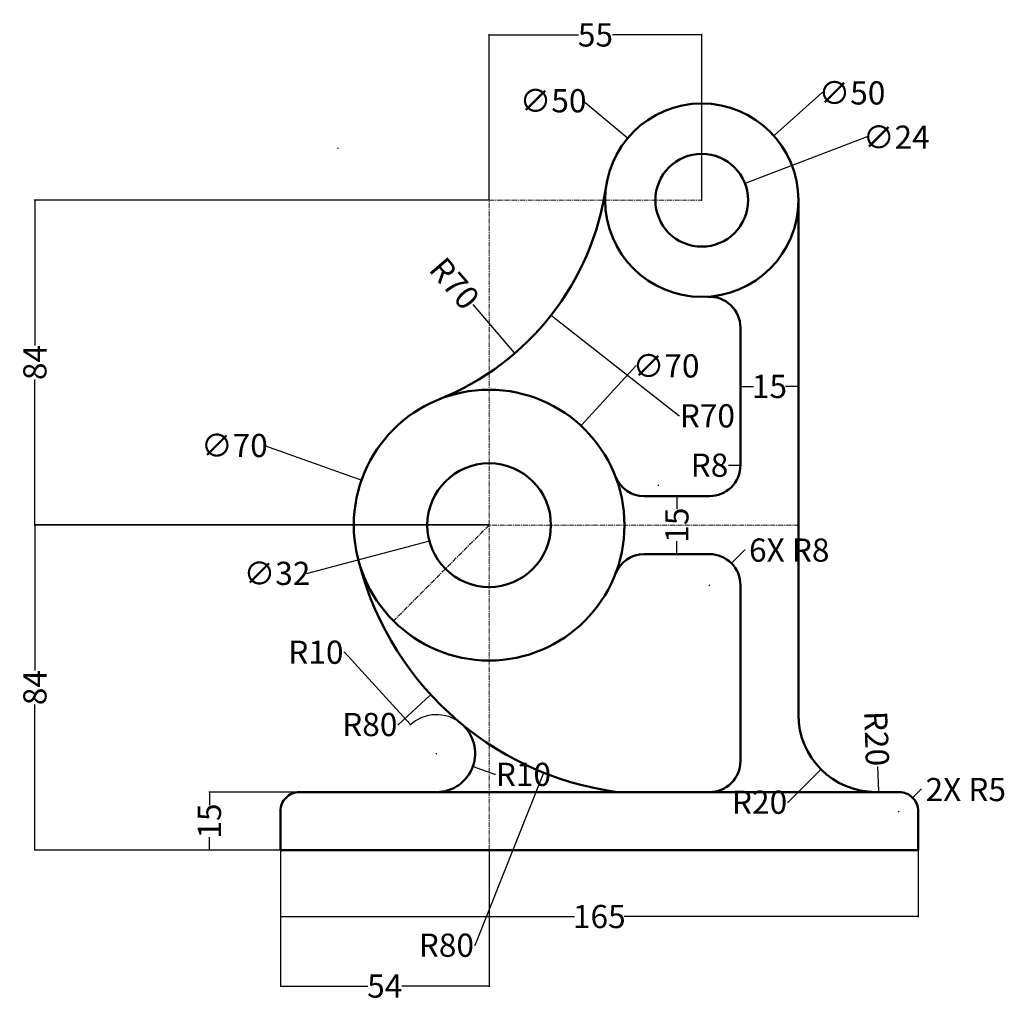
# Model space of a CAD drawing. Units: millimetres. Extents: x -55 to 200, y -2 to 251.
import ezdxf

# ---------------------------------------------------------------- set-up
doc = ezdxf.new("R2010")
doc.units = ezdxf.units.MM
doc.header["$MEASUREMENT"] = 0
doc.linetypes.add('CENTER', pattern=[2, 1.25, -0.25, 0.25, -0.25])
for name, color, linetype, lineweight in [('M-CNTR', 4, 'CENTER', 18), ('M-DIMS', 2, 'Continuous', 25), ('M-OUTL', 7, 'Continuous', 50)]:
    doc.layers.add(name, color=color, linetype=linetype, lineweight=lineweight)
doc.styles.get("Standard").update_dxf_attribs({"font": 'arial.ttf'})
doc.dimstyles.get("Standard").update_dxf_attribs({"dimtxt": 6, "dimasz": 0.18, "dimexe": 0.18, "dimexo": 0.0625, "dimgap": 0.09, "dimtad": 0, "dimtoh": 1, "dimdec": 0, "dimzin": 0, "dimdsep": 46, "dimtxsty": 'Standard', "dimcen": 0.09, "dimadec": 0, "dimazin": 0, "dimtfac": 1, "dimtdec": 0, "dimtofl": 0, "dimtmove": 0, "dimatfit": 3, "dimfxl": 1, "dimtolj": 1, "dimtzin": 0, "dimarcsym": 0})

# ---------------------------------------------------------------- blocks, each defined once
blk = doc.blocks.new('*D1')
at = {"layer": 'Defpoints', "color": 0, "transparency": 16777216}
for p in [(12.77, 36.84), (66.77, 36.84), (66.77, 1.69)]:
    blk.add_point(p, dxfattribs=at)
at = {"layer": 'M-DIMS', "color": 0, "lineweight": -2, "transparency": 16777216}
for p, q in [((12.77, 36.77), (12.77, 1.51)), ((66.77, 36.77), (66.77, 1.51)), ((12.95, 1.69), (35.4, 1.69)), ((66.59, 1.69), (44.15, 1.69))]:
    blk.add_line(p, q, dxfattribs=at)
at = {"layer": 'M-DIMS', "color": 0, "transparency": 16777216}
for points in [[(12.95, 1.72), (12.95, 1.66), (12.77, 1.69)], [(66.59, 1.72), (66.59, 1.66), (66.77, 1.69)]]:
    blk.add_solid(points, dxfattribs=at)
at = {"layer": 'M-DIMS', "color": 0, "transparency": 16777216, "insert": (39.77, 1.69), "char_height": 6, "attachment_point": 5}
blk.add_mtext('\\A1;54', dxfattribs=at)
blk = doc.blocks.new('*D2')
at = {"layer": 'Defpoints', "color": 0, "transparency": 16777216}
for p in [(123.77, 136.34), (131.77, 136.34)]:
    blk.add_point(p, dxfattribs=at)
at = {"layer": 'M-DIMS', "color": 0, "lineweight": -2, "transparency": 16777216}
blk.add_line((128.71, 136.34), (131.59, 136.34), dxfattribs=at)
blk.add_arc((123.77, 136.34), 8, 0.4476, 1.2892, dxfattribs=at)
at = {"layer": 'M-DIMS', "color": 0, "transparency": 16777216}
blk.add_solid([(131.59, 136.37), (131.59, 136.31), (131.77, 136.34)], dxfattribs=at)
at = {"layer": 'M-DIMS', "color": 0, "transparency": 16777216, "insert": (123.77, 136.34), "char_height": 6, "attachment_point": 5}
blk.add_mtext('\\A1;R8', dxfattribs=at)
blk = doc.blocks.new('*D3')
at = {"layer": 'Defpoints', "color": 0, "transparency": 16777216}
for p in [(27.73, 218.31), (73.38, 165.24)]:
    blk.add_point(p, dxfattribs=at)
at = {"layer": 'M-DIMS', "color": 0, "lineweight": -2, "transparency": 16777216}
blk.add_line((62.55, 177.84), (73.27, 165.38), dxfattribs=at)
at = {"layer": 'M-DIMS', "color": 0, "transparency": 16777216}
blk.add_solid([(73.29, 165.4), (73.24, 165.36), (73.38, 165.24)], dxfattribs=at)
at = {"layer": 'M-DIMS', "color": 0, "transparency": 16777216, "insert": (57.82, 183.33), "char_height": 6, "attachment_point": 5, "rotation": 310.7032}
blk.add_mtext('\\A1;R70', dxfattribs=at)
blk = doc.blocks.new('*D4')
at = {"layer": 'Defpoints', "color": 0, "transparency": 16777216}
for p in [(110.59, 131.13), (51.69, 76.99)]:
    blk.add_point(p, dxfattribs=at)
at = {"layer": 'M-DIMS', "color": 0, "lineweight": -2, "transparency": 16777216}
for p, q in [((110.5, 131.13), (110.68, 131.13)), ((110.59, 131.04), (110.59, 131.22)), ((43.33, 69.3), (51.56, 76.87)), ((43.15, 69.3), (43.33, 69.3))]:
    blk.add_line(p, q, dxfattribs=at)
at = {"layer": 'M-DIMS', "color": 0, "transparency": 16777216}
blk.add_solid([(51.54, 76.89), (51.58, 76.85), (51.69, 76.99)], dxfattribs=at)
at = {"layer": 'M-DIMS', "color": 0, "transparency": 16777216, "insert": (35.9, 69.3), "char_height": 6, "attachment_point": 5}
blk.add_mtext('\\A1;R80', dxfattribs=at)
blk = doc.blocks.new('*D5')
at = {"layer": 'Defpoints', "color": 0, "transparency": 16777216}
for p in [(46.43, 69.24), (53.16, 61.84)]:
    blk.add_point(p, dxfattribs=at)
at = {"layer": 'M-DIMS', "color": 0, "lineweight": -2, "transparency": 16777216}
for p, q in [((29.2, 87.99), (29.38, 87.99)), ((29.38, 87.99), (46.31, 69.37)), ((53.07, 61.84), (53.25, 61.84)), ((53.16, 61.75), (53.16, 61.93))]:
    blk.add_line(p, q, dxfattribs=at)
blk.add_arc((53.16, 61.84), 10, 50.7056, 133.3049, dxfattribs=at)
at = {"layer": 'M-DIMS', "color": 0, "transparency": 16777216}
blk.add_solid([(46.33, 69.39), (46.29, 69.35), (46.43, 69.24)], dxfattribs=at)
at = {"layer": 'M-DIMS', "color": 0, "transparency": 16777216, "insert": (21.96, 87.99), "char_height": 6, "attachment_point": 5}
blk.add_mtext('\\A1;R10', dxfattribs=at)
blk = doc.blocks.new('*D6')
at = {"layer": 'Defpoints', "color": 0, "transparency": 16777216}
for p in [(82.24, 124.92), (51.3, 116.75)]:
    blk.add_point(p, dxfattribs=at)
at = {"layer": 'M-DIMS', "color": 0, "lineweight": -2, "transparency": 16777216}
for p, q in [((66.68, 120.84), (66.86, 120.84)), ((66.77, 120.75), (66.77, 120.93)), ((19.52, 108.37), (51.13, 116.71))]:
    blk.add_line(p, q, dxfattribs=at)
at = {"layer": 'M-DIMS', "color": 0, "transparency": 16777216}
blk.add_solid([(51.12, 116.74), (51.14, 116.68), (51.3, 116.75)], dxfattribs=at)
at = {"layer": 'M-DIMS', "color": 0, "transparency": 16777216, "insert": (11.9, 108.37), "char_height": 6, "attachment_point": 5}
blk.add_mtext('\\A1;∅32', dxfattribs=at)
blk = doc.blocks.new('*D7')
at = {"layer": 'Defpoints', "color": 0, "transparency": 16777216}
for p in [(33.79, 132.53), (99.76, 109.14)]:
    blk.add_point(p, dxfattribs=at)
at = {"layer": 'M-DIMS', "color": 0, "lineweight": -2, "transparency": 16777216}
for p, q in [((8.52, 141.43), (8.7, 141.43)), ((8.7, 141.43), (33.62, 132.59)), ((66.68, 120.84), (66.86, 120.84)), ((66.77, 120.75), (66.77, 120.93))]:
    blk.add_line(p, q, dxfattribs=at)
at = {"layer": 'M-DIMS', "color": 0, "transparency": 16777216}
blk.add_solid([(33.63, 132.62), (33.61, 132.56), (33.79, 132.53)], dxfattribs=at)
at = {"layer": 'M-DIMS', "color": 0, "transparency": 16777216, "insert": (0.88, 141.43), "char_height": 6, "attachment_point": 5}
blk.add_mtext('\\A1;∅70', dxfattribs=at)
blk = doc.blocks.new('*D8')
at = {"layer": 'Defpoints', "color": 0, "transparency": 16777216}
for p in [(132.98, 209.13), (110.57, 200.54)]:
    blk.add_point(p, dxfattribs=at)
at = {"layer": 'M-DIMS', "color": 0, "lineweight": -2, "transparency": 16777216}
for p, q in [((164.28, 221.13), (133.15, 209.2)), ((164.46, 221.13), (164.28, 221.13)), ((121.68, 204.84), (121.86, 204.84)), ((121.77, 204.75), (121.77, 204.93))]:
    blk.add_line(p, q, dxfattribs=at)
at = {"layer": 'M-DIMS', "color": 0, "transparency": 16777216}
blk.add_solid([(133.14, 209.22), (133.16, 209.17), (132.98, 209.13)], dxfattribs=at)
at = {"layer": 'M-DIMS', "color": 0, "transparency": 16777216, "insert": (172.1, 221.13), "char_height": 6, "attachment_point": 5}
blk.add_mtext('\\A1;∅24', dxfattribs=at)
blk = doc.blocks.new('*D9')
at = {"layer": 'Defpoints', "color": 0, "transparency": 16777216}
for p in [(140.41, 221.5), (103.14, 188.17)]:
    blk.add_point(p, dxfattribs=at)
at = {"layer": 'M-DIMS', "color": 0, "lineweight": -2, "transparency": 16777216}
for p, q in [((152.81, 232.58), (140.55, 221.62)), ((152.99, 232.58), (152.81, 232.58)), ((121.68, 204.84), (121.86, 204.84)), ((121.77, 204.75), (121.77, 204.93))]:
    blk.add_line(p, q, dxfattribs=at)
at = {"layer": 'M-DIMS', "color": 0, "transparency": 16777216}
blk.add_solid([(140.53, 221.64), (140.57, 221.59), (140.41, 221.5)], dxfattribs=at)
at = {"layer": 'M-DIMS', "color": 0, "transparency": 16777216, "insert": (160.63, 232.58), "char_height": 6, "attachment_point": 5}
blk.add_mtext('\\A1;∅50', dxfattribs=at)
blk = doc.blocks.new('*D10')
at = {"layer": 'Defpoints', "color": 0, "transparency": 16777216}
for p in [(166.77, 71.84), (167.51, 51.85)]:
    blk.add_point(p, dxfattribs=at)
at = {"layer": 'M-DIMS', "color": 0, "lineweight": -2, "transparency": 16777216}
blk.add_line((167.27, 58.43), (167.51, 52.03), dxfattribs=at)
blk.add_arc((166.77, 71.84), 20, 270.179, 272.6379, dxfattribs=at)
at = {"layer": 'M-DIMS', "color": 0, "transparency": 16777216}
blk.add_solid([(167.54, 52.03), (167.48, 52.03), (167.51, 51.85)], dxfattribs=at)
at = {"layer": 'M-DIMS', "color": 0, "transparency": 16777216, "insert": (167, 65.67), "char_height": 6, "attachment_point": 5, "rotation": 272.1222}
blk.add_mtext('\\A1;R20', dxfattribs=at)
blk = doc.blocks.new('*D11')
at = {"layer": 'Defpoints', "color": 0, "transparency": 16777216}
for p in [(115.33, 128.34), (115.33, 113.34), (115.33, 113.34)]:
    blk.add_point(p, dxfattribs=at)
at = {"layer": 'M-DIMS', "color": 0, "lineweight": -2, "transparency": 16777216}
for p, q in [((115.33, 128.16), (115.33, 124.96)), ((115.39, 128.34), (115.51, 128.34)), ((115.33, 113.52), (115.33, 116.71)), ((115.39, 113.34), (115.51, 113.34))]:
    blk.add_line(p, q, dxfattribs=at)
at = {"layer": 'M-DIMS', "color": 0, "transparency": 16777216}
for points in [[(115.3, 128.16), (115.36, 128.16), (115.33, 128.34)], [(115.3, 113.52), (115.36, 113.52), (115.33, 113.34)]]:
    blk.add_solid(points, dxfattribs=at)
at = {"layer": 'M-DIMS', "color": 0, "transparency": 16777216, "insert": (115.33, 120.84), "char_height": 6, "attachment_point": 5, "rotation": 90}
blk.add_mtext('\\A1;15', dxfattribs=at)
blk = doc.blocks.new('*D12')
at = {"layer": 'Defpoints', "color": 0, "transparency": 16777216}
for p in [(131.77, 171.9), (146.77, 172.16), (146.77, 156.71)]:
    blk.add_point(p, dxfattribs=at)
at = {"layer": 'M-DIMS', "color": 0, "lineweight": -2, "transparency": 16777216}
for p, q in [((131.77, 171.83), (131.77, 156.53)), ((146.77, 172.1), (146.77, 156.53)), ((131.95, 156.71), (135.15, 156.71)), ((146.59, 156.71), (143.4, 156.71))]:
    blk.add_line(p, q, dxfattribs=at)
at = {"layer": 'M-DIMS', "color": 0, "transparency": 16777216}
for points in [[(131.95, 156.74), (131.95, 156.68), (131.77, 156.71)], [(146.59, 156.74), (146.59, 156.68), (146.77, 156.71)]]:
    blk.add_solid(points, dxfattribs=at)
at = {"layer": 'M-DIMS', "color": 0, "transparency": 16777216, "insert": (139.27, 156.71), "char_height": 6, "attachment_point": 5}
blk.add_mtext('\\A1;15', dxfattribs=at)
blk = doc.blocks.new('*D13')
at = {"layer": 'Defpoints', "color": 0, "transparency": 16777216}
for p in [(12.77, 36.84), (177.77, 36.84), (177.77, 19.67)]:
    blk.add_point(p, dxfattribs=at)
at = {"layer": 'M-DIMS', "color": 0, "lineweight": -2, "transparency": 16777216}
for p, q in [((12.77, 36.77), (12.77, 19.49)), ((177.77, 36.77), (177.77, 19.49)), ((12.95, 19.67), (88.82, 19.67)), ((177.59, 19.67), (101.73, 19.67))]:
    blk.add_line(p, q, dxfattribs=at)
at = {"layer": 'M-DIMS', "color": 0, "transparency": 16777216}
for points in [[(12.95, 19.7), (12.95, 19.64), (12.77, 19.67)], [(177.59, 19.7), (177.59, 19.64), (177.77, 19.67)]]:
    blk.add_solid(points, dxfattribs=at)
at = {"layer": 'M-DIMS', "color": 0, "transparency": 16777216, "insert": (95.27, 19.67), "char_height": 6, "attachment_point": 5}
blk.add_mtext('\\A1;165', dxfattribs=at)
blk = doc.blocks.new('*D14')
at = {"layer": 'Defpoints', "color": 0, "transparency": 16777216}
for p in [(-50.72, 120.84), (66.86, 120.84), (66.77, 36.84)]:
    blk.add_point(p, dxfattribs=at)
at = {"layer": 'M-DIMS', "color": 0, "lineweight": -2, "transparency": 16777216}
for p, q in [((66.8, 120.84), (-50.9, 120.84)), ((-50.72, 120.66), (-50.72, 83.22)), ((-50.72, 37.02), (-50.72, 74.46)), ((66.71, 36.84), (-50.9, 36.84))]:
    blk.add_line(p, q, dxfattribs=at)
at = {"layer": 'M-DIMS', "color": 0, "transparency": 16777216}
for points in [[(-50.75, 120.66), (-50.69, 120.66), (-50.72, 120.84)], [(-50.75, 37.02), (-50.69, 37.02), (-50.72, 36.84)]]:
    blk.add_solid(points, dxfattribs=at)
at = {"layer": 'M-DIMS', "color": 0, "transparency": 16777216, "insert": (-50.72, 78.84), "char_height": 6, "attachment_point": 5, "rotation": 90}
blk.add_mtext('\\A1;84', dxfattribs=at)
blk = doc.blocks.new('*D15')
at = {"layer": 'Defpoints', "color": 0, "transparency": 16777216}
for p in [(-50.72, 204.84), (66.77, 204.84), (66.77, 120.93)]:
    blk.add_point(p, dxfattribs=at)
at = {"layer": 'M-DIMS', "color": 0, "lineweight": -2, "transparency": 16777216}
for p, q in [((66.71, 204.84), (-50.9, 204.84)), ((-50.72, 204.66), (-50.72, 167.26)), ((-50.72, 121.11), (-50.72, 158.5)), ((66.71, 120.93), (-50.9, 120.93))]:
    blk.add_line(p, q, dxfattribs=at)
at = {"layer": 'M-DIMS', "color": 0, "transparency": 16777216}
for points in [[(-50.75, 204.66), (-50.69, 204.66), (-50.72, 204.84)], [(-50.75, 121.11), (-50.69, 121.11), (-50.72, 120.93)]]:
    blk.add_solid(points, dxfattribs=at)
at = {"layer": 'M-DIMS', "color": 0, "transparency": 16777216, "insert": (-50.72, 162.88), "char_height": 6, "attachment_point": 5, "rotation": 90}
blk.add_mtext('\\A1;84', dxfattribs=at)
blk = doc.blocks.new('*D16')
at = {"layer": 'Defpoints', "color": 0, "transparency": 16777216}
for p in [(121.77, 247.56), (66.77, 204.84), (121.77, 204.93)]:
    blk.add_point(p, dxfattribs=at)
at = {"layer": 'M-DIMS', "color": 0, "lineweight": -2, "transparency": 16777216}
for p, q in [((66.77, 204.9), (66.77, 247.74)), ((66.95, 247.56), (89.86, 247.56)), ((121.59, 247.56), (98.68, 247.56)), ((121.77, 204.99), (121.77, 247.74))]:
    blk.add_line(p, q, dxfattribs=at)
at = {"layer": 'M-DIMS', "color": 0, "transparency": 16777216}
for points in [[(66.95, 247.59), (66.95, 247.53), (66.77, 247.56)], [(121.59, 247.59), (121.59, 247.53), (121.77, 247.56)]]:
    blk.add_solid(points, dxfattribs=at)
at = {"layer": 'M-DIMS', "color": 0, "transparency": 16777216, "insert": (94.27, 247.56), "char_height": 6, "attachment_point": 5}
blk.add_mtext('\\A1;55', dxfattribs=at)
blk = doc.blocks.new('*D17')
at = {"layer": 'Defpoints', "color": 0, "transparency": 16777216}
for p in [(-5.58, 51.84), (17.77, 51.84), (12.77, 36.84)]:
    blk.add_point(p, dxfattribs=at)
at = {"layer": 'M-DIMS', "color": 0, "lineweight": -2, "transparency": 16777216}
for p, q in [((17.71, 51.84), (-5.76, 51.84)), ((-5.58, 51.66), (-5.58, 48.46)), ((-5.58, 37.02), (-5.58, 40.21)), ((12.71, 36.84), (-5.76, 36.84))]:
    blk.add_line(p, q, dxfattribs=at)
at = {"layer": 'M-DIMS', "color": 0, "transparency": 16777216}
for points in [[(-5.61, 51.66), (-5.55, 51.66), (-5.58, 51.84)], [(-5.61, 37.02), (-5.55, 37.02), (-5.58, 36.84)]]:
    blk.add_solid(points, dxfattribs=at)
at = {"layer": 'M-DIMS', "color": 0, "transparency": 16777216, "insert": (-5.58, 44.34), "char_height": 6, "attachment_point": 5, "rotation": 90}
blk.add_mtext('\\A1;15', dxfattribs=at)
blk = doc.blocks.new('*D18')
at = {"layer": 'Defpoints', "color": 0, "transparency": 16777216}
for p in [(90.5, 146.57), (43.05, 95.1)]:
    blk.add_point(p, dxfattribs=at)
at = {"layer": 'M-DIMS', "color": 0, "lineweight": -2, "transparency": 16777216}
for p, q in [((104.73, 162.01), (90.62, 146.7)), ((104.91, 162.01), (104.73, 162.01)), ((66.68, 120.84), (66.86, 120.84)), ((66.77, 120.75), (66.77, 120.93))]:
    blk.add_line(p, q, dxfattribs=at)
at = {"layer": 'M-DIMS', "color": 0, "transparency": 16777216}
blk.add_solid([(90.6, 146.72), (90.64, 146.68), (90.5, 146.57)], dxfattribs=at)
at = {"layer": 'M-DIMS', "color": 0, "transparency": 16777216, "insert": (112.55, 162.01), "char_height": 6, "attachment_point": 5}
blk.add_mtext('\\A1;∅70', dxfattribs=at)
blk = doc.blocks.new('*D19')
at = {"layer": 'Defpoints', "color": 0, "transparency": 16777216}
for p in [(102.62, 220.91), (140.92, 188.77)]:
    blk.add_point(p, dxfattribs=at)
at = {"layer": 'M-DIMS', "color": 0, "lineweight": -2, "transparency": 16777216}
for p, q in [((90.95, 230.55), (91.13, 230.55)), ((91.13, 230.55), (102.49, 221.02)), ((121.68, 204.84), (121.86, 204.84)), ((121.77, 204.75), (121.77, 204.93))]:
    blk.add_line(p, q, dxfattribs=at)
at = {"layer": 'M-DIMS', "color": 0, "transparency": 16777216}
blk.add_solid([(102.5, 221.04), (102.47, 221), (102.62, 220.91)], dxfattribs=at)
at = {"layer": 'M-DIMS', "color": 0, "transparency": 16777216, "insert": (83.31, 230.55), "char_height": 6, "attachment_point": 5}
blk.add_mtext('\\A1;∅50', dxfattribs=at)
blk = doc.blocks.new('*D20')
at = {"layer": 'Defpoints', "color": 0, "transparency": 16777216}
for p in [(110.59, 131.13), (80.93, 56.83)]:
    blk.add_point(p, dxfattribs=at)
at = {"layer": 'M-DIMS', "color": 0, "lineweight": -2, "transparency": 16777216}
for p, q in [((110.5, 131.13), (110.68, 131.13)), ((110.59, 131.04), (110.59, 131.22)), ((63.14, 12.25), (80.87, 56.66)), ((62.96, 12.25), (63.14, 12.25))]:
    blk.add_line(p, q, dxfattribs=at)
at = {"layer": 'M-DIMS', "color": 0, "transparency": 16777216}
blk.add_solid([(80.84, 56.67), (80.89, 56.65), (80.93, 56.83)], dxfattribs=at)
at = {"layer": 'M-DIMS', "color": 0, "transparency": 16777216, "insert": (55.71, 12.25), "char_height": 6, "attachment_point": 5}
blk.add_mtext('\\A1;R80', dxfattribs=at)
blk = doc.blocks.new('*D21')
at = {"layer": 'Defpoints', "color": 0, "transparency": 16777216}
for p in [(27.73, 218.31), (82.77, 175.06)]:
    blk.add_point(p, dxfattribs=at)
at = {"layer": 'M-DIMS', "color": 0, "lineweight": -2, "transparency": 16777216}
for p, q in [((27.64, 218.31), (27.82, 218.31)), ((27.73, 218.22), (27.73, 218.4)), ((115.8, 149.1), (82.91, 174.94)), ((115.98, 149.1), (115.8, 149.1))]:
    blk.add_line(p, q, dxfattribs=at)
at = {"layer": 'M-DIMS', "color": 0, "transparency": 16777216}
blk.add_solid([(82.93, 174.97), (82.9, 174.92), (82.77, 175.06)], dxfattribs=at)
at = {"layer": 'M-DIMS', "color": 0, "transparency": 16777216, "insert": (123.22, 149.1), "char_height": 6, "attachment_point": 5}
blk.add_mtext('\\A1;R70', dxfattribs=at)
blk = doc.blocks.new('*D22')
at = {"layer": 'Defpoints', "color": 0, "transparency": 16777216}
for p in [(166.77, 71.84), (152.63, 57.69)]:
    blk.add_point(p, dxfattribs=at)
at = {"layer": 'M-DIMS', "color": 0, "lineweight": -2, "transparency": 16777216}
for p, q in [((166.68, 71.84), (166.86, 71.84)), ((166.77, 71.75), (166.77, 71.93)), ((144.15, 49.21), (152.5, 57.57)), ((143.97, 49.21), (144.15, 49.21))]:
    blk.add_line(p, q, dxfattribs=at)
at = {"layer": 'M-DIMS', "color": 0, "transparency": 16777216}
blk.add_solid([(152.48, 57.59), (152.53, 57.55), (152.63, 57.69)], dxfattribs=at)
at = {"layer": 'M-DIMS', "color": 0, "transparency": 16777216, "insert": (136.72, 49.21), "char_height": 6, "attachment_point": 5}
blk.add_mtext('\\A1;R20', dxfattribs=at)
blk = doc.blocks.new('*D23')
at = {"layer": 'Defpoints', "color": 0, "transparency": 16777216}
for p in [(53.16, 61.84), (62.56, 58.44)]:
    blk.add_point(p, dxfattribs=at)
at = {"layer": 'M-DIMS', "color": 0, "lineweight": -2, "transparency": 16777216}
for p, q in [((53.07, 61.84), (53.25, 61.84)), ((53.16, 61.75), (53.16, 61.93)), ((68.21, 56.41), (62.73, 58.38)), ((68.39, 56.41), (68.21, 56.41))]:
    blk.add_line(p, q, dxfattribs=at)
at = {"layer": 'M-DIMS', "color": 0, "transparency": 16777216}
blk.add_solid([(62.74, 58.41), (62.72, 58.35), (62.56, 58.44)], dxfattribs=at)
at = {"layer": 'M-DIMS', "color": 0, "transparency": 16777216, "insert": (75.64, 56.41), "char_height": 6, "attachment_point": 5}
blk.add_mtext('\\A1;R10', dxfattribs=at)
blk = doc.blocks.new('*D24')
at = {"layer": 'Defpoints', "color": 0, "transparency": 16777216}
for p in [(129.43, 110.99), (123.77, 105.34)]:
    blk.add_point(p, dxfattribs=at)
at = {"layer": 'M-DIMS', "color": 0, "lineweight": -2, "transparency": 16777216}
for p, q in [((132.83, 114.39), (129.56, 111.12)), ((133.01, 114.39), (132.83, 114.39)), ((123.68, 105.34), (123.86, 105.34)), ((123.77, 105.25), (123.77, 105.43))]:
    blk.add_line(p, q, dxfattribs=at)
at = {"layer": 'M-DIMS', "color": 0, "transparency": 16777216}
blk.add_solid([(129.54, 111.14), (129.58, 111.1), (129.43, 110.99)], dxfattribs=at)
at = {"layer": 'M-DIMS', "color": 0, "transparency": 16777216, "insert": (144.4, 114.39), "char_height": 6, "attachment_point": 5}
blk.add_mtext('\\A1;6X R8', dxfattribs=at)
blk = doc.blocks.new('*D25')
at = {"layer": 'Defpoints', "color": 0, "transparency": 16777216}
for p in [(176.31, 50.37), (172.77, 46.84)]:
    blk.add_point(p, dxfattribs=at)
at = {"layer": 'M-DIMS', "color": 0, "lineweight": -2, "transparency": 16777216}
for p, q in [((178.43, 52.49), (176.44, 50.5)), ((178.61, 52.49), (178.43, 52.49)), ((172.68, 46.84), (172.86, 46.84)), ((172.77, 46.75), (172.77, 46.93))]:
    blk.add_line(p, q, dxfattribs=at)
at = {"layer": 'M-DIMS', "color": 0, "transparency": 16777216}
blk.add_solid([(176.42, 50.52), (176.46, 50.48), (176.31, 50.37)], dxfattribs=at)
at = {"layer": 'M-DIMS', "color": 0, "transparency": 16777216, "insert": (190.06, 52.49), "char_height": 6, "attachment_point": 5}
blk.add_mtext('\\A1;2X R5', dxfattribs=at)

msp = doc.modelspace()

# ---------------------------------------------------------------- linework, layer by layer
at = {"layer": 'M-CNTR'}
for points in [[(66.77, 19.14), (66.77, 36.84), (66.77, 120.84), (66.77, 204.84), (121.77, 204.84)], [(146.77, 120.84), (66.77, 120.84), (42.03, 96.09)]]:
    msp.add_lwpolyline(points, dxfattribs=at)
at = {"layer": 'M-OUTL'}
msp.add_line((146.77, 204.84), (146.77, 71.84), dxfattribs=at)
for points in [[(131.77, 136.34), (131.77, 171.9, 0.432089), (123.29, 179.88)], [(99.42, 133.45, 0.309892), (106.88, 128.34), (123.77, 128.34, 0.414214), (131.77, 136.34)], [(131.77, 105.34, 0.414214), (123.77, 113.34), (106.88, 113.34, 0.309892), (99.42, 108.22)], [(123.77, 51.84, 0.414214), (131.77, 59.84), (131.77, 105.34)]]:
    msp.add_lwpolyline(points, format="xyb", dxfattribs=at)
msp.add_lwpolyline([(177.77, 36.84), (177.77, 46.84, 0.414214), (172.77, 51.84), (166.77, 51.84), (17.77, 51.84, 0.414214), (12.77, 46.84), (12.77, 36.84)], format="xyb", close=True, dxfattribs=at)
for centre, radius in [((121.77, 204.84), 25), ((121.77, 204.84), 12), ((66.77, 120.84), 35), ((66.77, 120.84), 16)]:
    msp.add_circle(centre, radius, dxfattribs=at)
for centre, radius, start, end in [((27.73, 218.31), 70, 291.8272, 351.8471), ((110.59, 131.13), 80, 192.5253, 262.3803), ((166.77, 71.84), 20, 180, 270), ((53.16, 61.84), 10, 270, 50.3475)]:
    msp.add_arc(centre, radius, start, end, dxfattribs=at)

# ---------------------------------------------------------------- dimensions: what is measured, and where the dimension line sits
at = {"layer": 'M-DIMS'}
for base, p1, p2, picture, middle in [((121.77, 247.56), (66.77, 204.84), (121.77, 204.93), '*D16', (94.27, 247.56)), ((146.77, 156.71), (131.77, 171.9), (146.77, 172.16), '*D12', (139.27, 156.71)), ((66.77, 1.69), (12.77, 36.84), (66.77, 36.84), '*D1', (39.77, 1.69)), ((177.77, 19.67), (12.77, 36.84), (177.77, 36.84), '*D13', (95.27, 19.67))]:
    dim = msp.add_linear_dim(base=base, p1=p1, p2=p2, dimstyle='Standard', override={"dimclrd": 0, "dimclre": 0, "dimclrt": 0}, dxfattribs=at)
    dim.commit()
    dim.dimension.update_dxf_attribs({"geometry": picture, "text_midpoint": middle})
for p1, p2, override, picture, middle in [((140.92, 188.77), (102.62, 220.91), {"dimdec": 0, "dimlfac": 1, "dimrnd": 0, "dimzin": 0, "dimdsep": 46, "dimlunit": 2}, '*D19', (83.31, 230.55)), ((103.14, 188.17), (140.41, 221.5), {"dimclrd": 0, "dimclre": 0, "dimclrt": 0}, '*D9', (160.63, 232.58)), ((110.57, 200.54), (132.98, 209.13), {"dimclrd": 0, "dimclre": 0, "dimclrt": 0}, '*D8', (172.1, 221.13)), ((43.05, 95.1), (90.5, 146.57), {"dimdec": 0, "dimlfac": 1, "dimrnd": 0, "dimzin": 0, "dimdsep": 46, "dimlunit": 2}, '*D18', (112.55, 162.01)), ((99.76, 109.14), (33.79, 132.53), {"dimclrd": 0, "dimclre": 0, "dimclrt": 0}, '*D7', (0.88, 141.43)), ((82.24, 124.92), (51.3, 116.75), {"dimclrd": 0, "dimclre": 0, "dimclrt": 0}, '*D6', (19.52, 108.37))]:
    dim = msp.add_diameter_dim_2p(p1=p1, p2=p2, dimstyle='Standard', override=override, dxfattribs=at)
    dim.commit()
    dim.dimension.update_dxf_attribs({"geometry": picture, "text_midpoint": middle, "dimtype": 163})
for center, mpoint, override, picture, middle in [((27.73, 218.31), (82.77, 175.06), {"dimdec": 0, "dimlfac": 1, "dimrnd": 0, "dimzin": 0, "dimdsep": 46, "dimlunit": 2}, '*D21', (123.22, 149.1)), ((27.73, 218.31), (73.38, 165.24), {"dimclrd": 0, "dimclre": 0, "dimclrt": 0}, '*D3', (57.82, 183.33)), ((123.77, 136.34), (131.77, 136.34), {"dimclrd": 0, "dimclre": 0, "dimclrt": 0}, '*D2', (123.77, 136.34)), ((110.59, 131.13), (51.69, 76.99), {"dimclrd": 0, "dimclre": 0, "dimclrt": 0}, '*D4', (35.9, 69.3)), ((110.59, 131.13), (80.93, 56.83), {"dimdec": 0, "dimlfac": 1, "dimrnd": 0, "dimzin": 0, "dimdsep": 46, "dimlunit": 2}, '*D20', (55.71, 12.25)), ((53.16, 61.84), (46.43, 69.24), {"dimclrd": 0, "dimclre": 0, "dimclrt": 0}, '*D5', (21.96, 87.99)), ((166.77, 71.84), (152.63, 57.69), {"dimdec": 0, "dimlfac": 1, "dimrnd": 0, "dimzin": 0, "dimdsep": 46, "dimlunit": 2}, '*D22', (136.72, 49.21)), ((166.77, 71.84), (167.51, 51.85), {"dimclrd": 0, "dimclre": 0, "dimclrt": 0}, '*D10', (167, 65.67)), ((53.16, 61.84), (62.56, 58.44), {"dimdec": 0, "dimlfac": 1, "dimrnd": 0, "dimzin": 0, "dimdsep": 46, "dimlunit": 2}, '*D23', (75.64, 56.41))]:
    dim = msp.add_radius_dim(center=center, mpoint=mpoint, dimstyle='Standard', override=override, dxfattribs=at)
    dim.commit()
    dim.dimension.update_dxf_attribs({"geometry": picture, "text_midpoint": middle, "dimtype": 164})
for base, p1, p2, override, picture, middle in [((-50.72, 204.84), (66.77, 120.93), (66.77, 204.84), {"dimclrd": 0, "dimclre": 0, "dimclrt": 0}, '*D15', (-50.72, 162.88)), ((115.33, 113.34), (115.33, 128.34), (115.33, 113.34), {"dimclrd": 0, "dimclre": 0, "dimclrt": 0}, '*D11', (115.33, 120.84)), ((-50.72, 120.84), (66.77, 36.84), (66.86, 120.84), {"dimclrd": 0, "dimclre": 0, "dimclrt": 0}, '*D14', (-50.72, 78.84)), ((-5.58, 51.84), (12.77, 36.84), (17.77, 51.84), {"dimdec": 0, "dimlfac": 1, "dimrnd": 0, "dimzin": 0, "dimdsep": 46, "dimlunit": 2}, '*D17', (-5.58, 44.34))]:
    dim = msp.add_linear_dim(base=base, p1=p1, p2=p2, angle=90, dimstyle='Standard', override=override, dxfattribs=at)
    dim.commit()
    dim.dimension.update_dxf_attribs({"geometry": picture, "text_midpoint": middle})
for center, mpoint, text, picture, middle in [((123.77, 105.34), (129.43, 110.99), '6X <>', '*D24', (144.4, 114.39)), ((172.77, 46.84), (176.31, 50.37), '2X <>', '*D25', (190.06, 52.49))]:
    dim = msp.add_radius_dim(center=center, mpoint=mpoint, text=text, dimstyle='Standard', override={"dimdec": 0, "dimlfac": 1, "dimrnd": 0, "dimzin": 0, "dimdsep": 46, "dimlunit": 2}, dxfattribs=at)
    dim.commit()
    dim.dimension.update_dxf_attribs({"geometry": picture, "text_midpoint": middle, "dimtype": 164})

doc.saveas('drawing.dxf')
